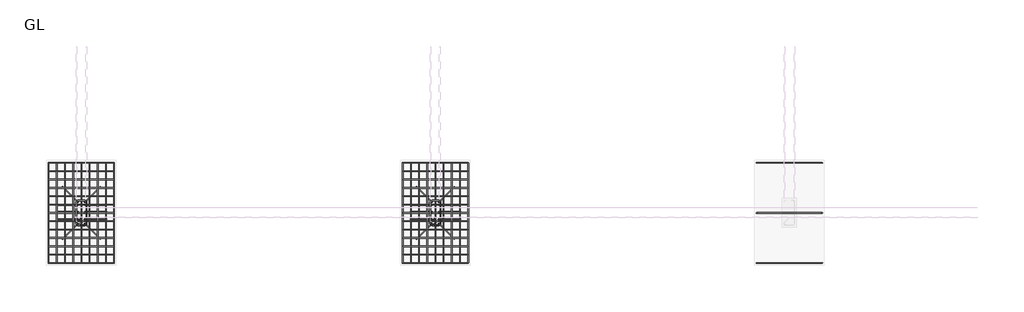
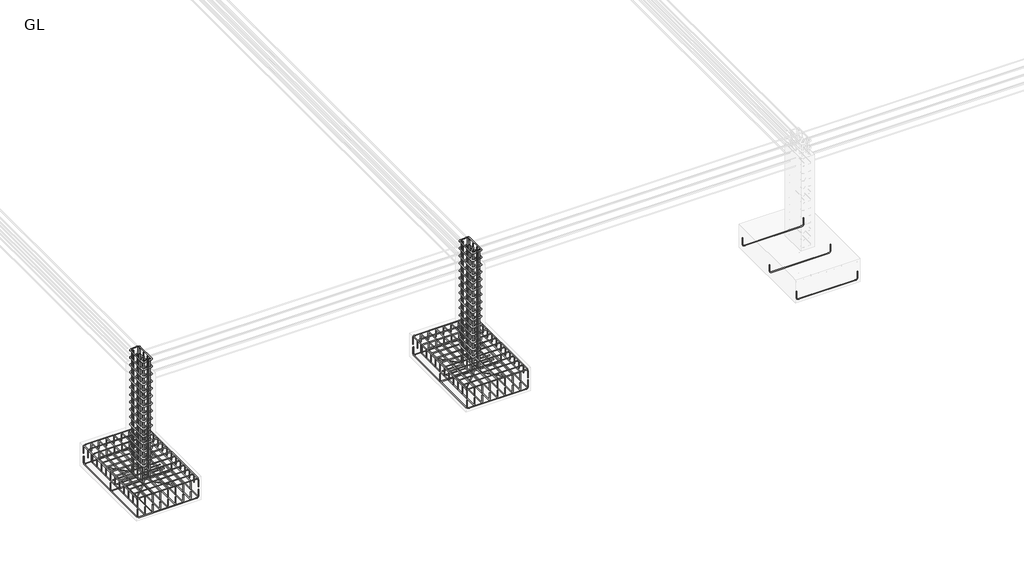
# One storey, part 2 of 16: 23 reinforcing bars.
"""IFC4 building model written with IfcOpenShell, lengths in millimetres."""

from ifc_helpers import new_model, si_unit, point, frame, origin, place, context, project, spatial, polyline, circle_curve, trimmed, segment, composite_curve, source, transform, mapped, element, save
from ifc_brep_helpers import swept_disk

model = new_model("IFC4")

# Units and contexts
model_context = context("Model", 3, world=origin())
ifc_project = project(units=[si_unit("LENGTHUNIT", "METRE", prefix="MILLI")], contexts=[model_context])

# Site, building, storey
site = spatial("IfcSite", under=ifc_project)
building = spatial("IfcBuilding", under=site)
storey = spatial("IfcBuildingStorey", under=building, Name="GL", Elevation=-1829.0)

# Reinforcing bars
placement = place(None, origin())
reinforcing_bar_shape = source(origin(), model_context, "Body", "SolidModel", [
    swept_disk(composite_curve([segment(polyline([(-22242.9544379, -19415.1167521, -2089.0), (-22242.9544379, -19415.1167521, -2213.0)]), True, "CONTINUOUS"), segment(trimmed(circle_curve(frame((-22272.9544379, -19415.1167521, -2213.0), z_axis=(0.0, 1.0, 0.0), x_axis=(30.0, 0.0, 0.0)), 30.0), [point((-22242.9544379, -19415.1167521, -2213.0))], [point((-22272.9544379, -19415.1167521, -2243.0))], True, "CARTESIAN"), True, "CONTINUOUS"), segment(polyline([(-22272.9544379, -19415.1167521, -2243.0), (-23340.9544379, -19415.1167521, -2243.0)]), True, "CONTINUOUS"), segment(trimmed(circle_curve(frame((-23340.9544379, -19415.1167521, -2213.0), z_axis=(0.0, 1.0, 0.0), x_axis=(0.0, 0.0, -30.0)), 30.0), [point((-23340.9544379, -19415.1167521, -2243.0))], [point((-23370.9544379, -19415.1167521, -2213.0))], True, "CARTESIAN"), True, "CONTINUOUS"), segment(polyline([(-23370.9544379, -19415.1167521, -2213.0), (-23370.9544379, -19415.1167521, -2089.0)]), True, "CONTINUOUS")], self_intersect=False), 6.0),
])
element("IfcReinforcingBar", 1, at=placement, inside=storey, context=model_context, shape_type="MappedRepresentation", body=[
    mapped(reinforcing_bar_shape, transform((0.0, 0.0, 0.0), x_axis=(1.0, 0.0, 0.0), y_axis=(0.0, 1.0, 0.0), z_axis=(0.0, 0.0, 1.0))),
    mapped(reinforcing_bar_shape, transform((0.0, -864.0, 0.0), x_axis=(1.0, 0.0, 0.0), y_axis=(0.0, 1.0, 0.0), z_axis=(0.0, 0.0, 1.0))),
    mapped(reinforcing_bar_shape, transform((0.0, -1728.0, 0.0), x_axis=(1.0, 0.0, 0.0), y_axis=(0.0, 1.0, 0.0), z_axis=(0.0, 0.0, 1.0))),
])
reinforcing_bar_2_shape = source(origin(), model_context, "Body", "SolidModel", [
    swept_disk(composite_curve([segment(polyline([(-23370.9544379, -19415.1167521, -2022.436678), (-23370.9544379, -19415.1167521, -1898.436678)]), True, "CONTINUOUS"), segment(trimmed(circle_curve(frame((-23340.9544379, -19415.1167521, -1898.436678), z_axis=(0.0, 1.0, 0.0), x_axis=(-30.0, 0.0, 0.0)), 30.0), [point((-23370.9544379, -19415.1167521, -1898.436678))], [point((-23340.9544379, -19415.1167521, -1868.436678))], True, "CARTESIAN"), True, "CONTINUOUS"), segment(polyline([(-23340.9544379, -19415.1167521, -1868.436678), (-22272.9544379, -19415.1167521, -1868.436678)]), True, "CONTINUOUS"), segment(trimmed(circle_curve(frame((-22272.9544379, -19415.1167521, -1898.436678), z_axis=(0.0, 1.0, 0.0), x_axis=(0.0, 0.0, 30.0)), 30.0), [point((-22272.9544379, -19415.1167521, -1868.436678))], [point((-22242.9544379, -19415.1167521, -1898.436678))], True, "CARTESIAN"), True, "CONTINUOUS"), segment(polyline([(-22242.9544379, -19415.1167521, -1898.436678), (-22242.9544379, -19415.1167521, -2022.436678)]), True, "CONTINUOUS")], self_intersect=False), 6.0),
])
element("IfcReinforcingBar", 2, at=placement, inside=storey, context=model_context, shape_type="MappedRepresentation", body=[
    mapped(reinforcing_bar_2_shape, transform((0.0, 0.0, 0.0), x_axis=(1.0, 0.0, 0.0), y_axis=(0.0, 1.0, 0.0), z_axis=(0.0, 0.0, 1.0))),
    mapped(reinforcing_bar_2_shape, transform((0.0, -144.0, 0.0), x_axis=(1.0, 0.0, 0.0), y_axis=(0.0, 1.0, 0.0), z_axis=(0.0, 0.0, 1.0))),
    mapped(reinforcing_bar_2_shape, transform((0.0, -288.0, 0.0), x_axis=(1.0, 0.0, 0.0), y_axis=(0.0, 1.0, 0.0), z_axis=(0.0, 0.0, 1.0))),
    mapped(reinforcing_bar_2_shape, transform((0.0, -432.0, 0.0), x_axis=(1.0, 0.0, 0.0), y_axis=(0.0, 1.0, 0.0), z_axis=(0.0, 0.0, 1.0))),
    mapped(reinforcing_bar_2_shape, transform((0.0, -576.0, 0.0), x_axis=(1.0, 0.0, 0.0), y_axis=(0.0, 1.0, 0.0), z_axis=(0.0, 0.0, 1.0))),
    mapped(reinforcing_bar_2_shape, transform((0.0, -720.0, 0.0), x_axis=(1.0, 0.0, 0.0), y_axis=(0.0, 1.0, 0.0), z_axis=(0.0, 0.0, 1.0))),
    mapped(reinforcing_bar_2_shape, transform((0.0, -864.0, 0.0), x_axis=(1.0, 0.0, 0.0), y_axis=(0.0, 1.0, 0.0), z_axis=(0.0, 0.0, 1.0))),
    mapped(reinforcing_bar_2_shape, transform((0.0, -1008.0, 0.0), x_axis=(1.0, 0.0, 0.0), y_axis=(0.0, 1.0, 0.0), z_axis=(0.0, 0.0, 1.0))),
    mapped(reinforcing_bar_2_shape, transform((0.0, -1152.0, 0.0), x_axis=(1.0, 0.0, 0.0), y_axis=(0.0, 1.0, 0.0), z_axis=(0.0, 0.0, 1.0))),
    mapped(reinforcing_bar_2_shape, transform((0.0, -1296.0, 0.0), x_axis=(1.0, 0.0, 0.0), y_axis=(0.0, 1.0, 0.0), z_axis=(0.0, 0.0, 1.0))),
    mapped(reinforcing_bar_2_shape, transform((0.0, -1440.0, 0.0), x_axis=(1.0, 0.0, 0.0), y_axis=(0.0, 1.0, 0.0), z_axis=(0.0, 0.0, 1.0))),
    mapped(reinforcing_bar_2_shape, transform((0.0, -1584.0, 0.0), x_axis=(1.0, 0.0, 0.0), y_axis=(0.0, 1.0, 0.0), z_axis=(0.0, 0.0, 1.0))),
    mapped(reinforcing_bar_2_shape, transform((0.0, -1728.0, 0.0), x_axis=(1.0, 0.0, 0.0), y_axis=(0.0, 1.0, 0.0), z_axis=(0.0, 0.0, 1.0))),
])
reinforcing_bar_3_shape = source(origin(), model_context, "Body", "SolidModel", [
    swept_disk(composite_curve([segment(polyline([(-23370.9544379, -21143.1167521, -2027.5081232), (-23370.9544379, -21143.1167521, -1903.5081232)]), True, "CONTINUOUS"), segment(trimmed(circle_curve(frame((-23370.9544379, -21113.1167521, -1903.5081232), z_axis=(-1.0, 0.0, 0.0), x_axis=(0.0, -30.0, 0.0)), 30.0), [point((-23370.9544379, -21143.1167521, -1903.5081232))], [point((-23370.9544379, -21113.1167521, -1873.5081232))], True, "CARTESIAN"), True, "CONTINUOUS"), segment(polyline([(-23370.9544379, -21113.1167521, -1873.5081232), (-23370.9544379, -19445.1167521, -1873.5081232)]), True, "CONTINUOUS"), segment(trimmed(circle_curve(frame((-23370.9544379, -19445.1167521, -1903.5081232), z_axis=(-1.0, 0.0, 0.0), x_axis=(0.0, 0.0, 30.0)), 30.0), [point((-23370.9544379, -19445.1167521, -1873.5081232))], [point((-23370.9544379, -19415.1167521, -1903.5081232))], True, "CARTESIAN"), True, "CONTINUOUS"), segment(polyline([(-23370.9544379, -19415.1167521, -1903.5081232), (-23370.9544379, -19415.1167521, -2027.5081232)]), True, "CONTINUOUS")], self_intersect=False), 6.0),
])
element("IfcReinforcingBar", 3, at=placement, inside=storey, context=model_context, shape_type="MappedRepresentation", body=[
    mapped(reinforcing_bar_3_shape, transform((0.0, 0.0, 0.0), x_axis=(1.0, 0.0, 0.0), y_axis=(0.0, 1.0, 0.0), z_axis=(0.0, 0.0, 1.0))),
    mapped(reinforcing_bar_3_shape, transform((141.0, 0.0, 0.0), x_axis=(1.0, 0.0, 0.0), y_axis=(0.0, 1.0, 0.0), z_axis=(0.0, 0.0, 1.0))),
    mapped(reinforcing_bar_3_shape, transform((282.0, 0.0, 0.0), x_axis=(1.0, 0.0, 0.0), y_axis=(0.0, 1.0, 0.0), z_axis=(0.0, 0.0, 1.0))),
    mapped(reinforcing_bar_3_shape, transform((423.0, 0.0, 0.0), x_axis=(1.0, 0.0, 0.0), y_axis=(0.0, 1.0, 0.0), z_axis=(0.0, 0.0, 1.0))),
    mapped(reinforcing_bar_3_shape, transform((564.0, 0.0, 0.0), x_axis=(1.0, 0.0, 0.0), y_axis=(0.0, 1.0, 0.0), z_axis=(0.0, 0.0, 1.0))),
    mapped(reinforcing_bar_3_shape, transform((705.0, 0.0, 0.0), x_axis=(1.0, 0.0, 0.0), y_axis=(0.0, 1.0, 0.0), z_axis=(0.0, 0.0, 1.0))),
    mapped(reinforcing_bar_3_shape, transform((846.0, 0.0, 0.0), x_axis=(1.0, 0.0, 0.0), y_axis=(0.0, 1.0, 0.0), z_axis=(0.0, 0.0, 1.0))),
    mapped(reinforcing_bar_3_shape, transform((987.0, 0.0, 0.0), x_axis=(1.0, 0.0, 0.0), y_axis=(0.0, 1.0, 0.0), z_axis=(0.0, 0.0, 1.0))),
    mapped(reinforcing_bar_3_shape, transform((1128.0, 0.0, 0.0), x_axis=(1.0, 0.0, 0.0), y_axis=(0.0, 1.0, 0.0), z_axis=(0.0, 0.0, 1.0))),
])
reinforcing_bar_4_shape = source(origin(), model_context, "Body", "SolidModel", [
    swept_disk(composite_curve([segment(polyline([(-22242.9544379, -21143.1167521, -2080.6239909), (-22242.9544379, -21143.1167521, -2204.6239909)]), True, "CONTINUOUS"), segment(trimmed(circle_curve(frame((-22242.9544379, -21113.1167521, -2204.6239909), z_axis=(1.0, 0.0, 0.0), x_axis=(0.0, -30.0, 0.0)), 30.0), [point((-22242.9544379, -21143.1167521, -2204.6239909))], [point((-22242.9544379, -21113.1167521, -2234.6239909))], True, "CARTESIAN"), True, "CONTINUOUS"), segment(polyline([(-22242.9544379, -21113.1167521, -2234.6239909), (-22242.9544379, -19458.1421892, -2234.6239909)]), True, "CONTINUOUS"), segment(trimmed(circle_curve(frame((-22242.9544379, -19458.1421892, -2204.6239909), z_axis=(1.0, 0.0, 0.0), x_axis=(0.0, 0.0, -30.0)), 30.0), [point((-22242.9544379, -19458.1421892, -2234.6239909))], [point((-22242.9544379, -19428.1421892, -2204.6239909))], True, "CARTESIAN"), True, "CONTINUOUS"), segment(polyline([(-22242.9544379, -19428.1421892, -2204.6239909), (-22242.9544379, -19428.1421892, -2080.6239909)]), True, "CONTINUOUS")], self_intersect=False), 6.0),
])
element("IfcReinforcingBar", 4, at=placement, inside=storey, context=model_context, shape_type="MappedRepresentation", body=[
    mapped(reinforcing_bar_4_shape, transform((0.0, 0.0, 0.0), x_axis=(1.0, 0.0, 0.0), y_axis=(0.0, 1.0, 0.0), z_axis=(0.0, 0.0, 1.0))),
    mapped(reinforcing_bar_4_shape, transform((-141.0, 0.0, 0.0), x_axis=(1.0, 0.0, 0.0), y_axis=(0.0, 1.0, 0.0), z_axis=(0.0, 0.0, 1.0))),
    mapped(reinforcing_bar_4_shape, transform((-282.0, 0.0, 0.0), x_axis=(1.0, 0.0, 0.0), y_axis=(0.0, 1.0, 0.0), z_axis=(0.0, 0.0, 1.0))),
    mapped(reinforcing_bar_4_shape, transform((-423.0, 0.0, 0.0), x_axis=(1.0, 0.0, 0.0), y_axis=(0.0, 1.0, 0.0), z_axis=(0.0, 0.0, 1.0))),
    mapped(reinforcing_bar_4_shape, transform((-564.0, 0.0, 0.0), x_axis=(1.0, 0.0, 0.0), y_axis=(0.0, 1.0, 0.0), z_axis=(0.0, 0.0, 1.0))),
    mapped(reinforcing_bar_4_shape, transform((-705.0, 0.0, 0.0), x_axis=(1.0, 0.0, 0.0), y_axis=(0.0, 1.0, 0.0), z_axis=(0.0, 0.0, 1.0))),
    mapped(reinforcing_bar_4_shape, transform((-846.0, 0.0, 0.0), x_axis=(1.0, 0.0, 0.0), y_axis=(0.0, 1.0, 0.0), z_axis=(0.0, 0.0, 1.0))),
    mapped(reinforcing_bar_4_shape, transform((-987.0, 0.0, 0.0), x_axis=(1.0, 0.0, 0.0), y_axis=(0.0, 1.0, 0.0), z_axis=(0.0, 0.0, 1.0))),
    mapped(reinforcing_bar_4_shape, transform((-1128.0, 0.0, 0.0), x_axis=(1.0, 0.0, 0.0), y_axis=(0.0, 1.0, 0.0), z_axis=(0.0, 0.0, 1.0))),
])
reinforcing_bar_5_shape = source(origin(), model_context, "Body", "SolidModel", [
    swept_disk(composite_curve([segment(polyline([(-16146.9544379, -19415.1167521, -2089.0), (-16146.9544379, -19415.1167521, -2213.0)]), True, "CONTINUOUS"), segment(trimmed(circle_curve(frame((-16176.9544379, -19415.1167521, -2213.0), z_axis=(0.0, 1.0, 0.0), x_axis=(30.0, 0.0, 0.0)), 30.0), [point((-16146.9544379, -19415.1167521, -2213.0))], [point((-16176.9544379, -19415.1167521, -2243.0))], True, "CARTESIAN"), True, "CONTINUOUS"), segment(polyline([(-16176.9544379, -19415.1167521, -2243.0), (-17244.9544379, -19415.1167521, -2243.0)]), True, "CONTINUOUS"), segment(trimmed(circle_curve(frame((-17244.9544379, -19415.1167521, -2213.0), z_axis=(0.0, 1.0, 0.0), x_axis=(0.0, 0.0, -30.0)), 30.0), [point((-17244.9544379, -19415.1167521, -2243.0))], [point((-17274.9544379, -19415.1167521, -2213.0))], True, "CARTESIAN"), True, "CONTINUOUS"), segment(polyline([(-17274.9544379, -19415.1167521, -2213.0), (-17274.9544379, -19415.1167521, -2089.0)]), True, "CONTINUOUS")], self_intersect=False), 6.0),
])
element("IfcReinforcingBar", 5, at=placement, inside=storey, context=model_context, shape_type="MappedRepresentation", body=[
    mapped(reinforcing_bar_5_shape, transform((0.0, 0.0, 0.0), x_axis=(1.0, 0.0, 0.0), y_axis=(0.0, 1.0, 0.0), z_axis=(0.0, 0.0, 1.0))),
    mapped(reinforcing_bar_5_shape, transform((0.0, -864.0, 0.0), x_axis=(1.0, 0.0, 0.0), y_axis=(0.0, 1.0, 0.0), z_axis=(0.0, 0.0, 1.0))),
    mapped(reinforcing_bar_5_shape, transform((0.0, -1728.0, 0.0), x_axis=(1.0, 0.0, 0.0), y_axis=(0.0, 1.0, 0.0), z_axis=(0.0, 0.0, 1.0))),
])
reinforcing_bar_6_shape = source(origin(), model_context, "Body", "SolidModel", [
    swept_disk(composite_curve([segment(polyline([(-17274.9544379, -19415.1167521, -2022.436678), (-17274.9544379, -19415.1167521, -1898.436678)]), True, "CONTINUOUS"), segment(trimmed(circle_curve(frame((-17244.9544379, -19415.1167521, -1898.436678), z_axis=(0.0, 1.0, 0.0), x_axis=(-30.0, 0.0, 0.0)), 30.0), [point((-17274.9544379, -19415.1167521, -1898.436678))], [point((-17244.9544379, -19415.1167521, -1868.436678))], True, "CARTESIAN"), True, "CONTINUOUS"), segment(polyline([(-17244.9544379, -19415.1167521, -1868.436678), (-16176.9544379, -19415.1167521, -1868.436678)]), True, "CONTINUOUS"), segment(trimmed(circle_curve(frame((-16176.9544379, -19415.1167521, -1898.436678), z_axis=(0.0, 1.0, 0.0), x_axis=(0.0, 0.0, 30.0)), 30.0), [point((-16176.9544379, -19415.1167521, -1868.436678))], [point((-16146.9544379, -19415.1167521, -1898.436678))], True, "CARTESIAN"), True, "CONTINUOUS"), segment(polyline([(-16146.9544379, -19415.1167521, -1898.436678), (-16146.9544379, -19415.1167521, -2022.436678)]), True, "CONTINUOUS")], self_intersect=False), 6.0),
])
element("IfcReinforcingBar", 6, at=placement, inside=storey, context=model_context, shape_type="MappedRepresentation", body=[
    mapped(reinforcing_bar_6_shape, transform((0.0, 0.0, 0.0), x_axis=(1.0, 0.0, 0.0), y_axis=(0.0, 1.0, 0.0), z_axis=(0.0, 0.0, 1.0))),
    mapped(reinforcing_bar_6_shape, transform((0.0, -144.0, 0.0), x_axis=(1.0, 0.0, 0.0), y_axis=(0.0, 1.0, 0.0), z_axis=(0.0, 0.0, 1.0))),
    mapped(reinforcing_bar_6_shape, transform((0.0, -288.0, 0.0), x_axis=(1.0, 0.0, 0.0), y_axis=(0.0, 1.0, 0.0), z_axis=(0.0, 0.0, 1.0))),
    mapped(reinforcing_bar_6_shape, transform((0.0, -432.0, 0.0), x_axis=(1.0, 0.0, 0.0), y_axis=(0.0, 1.0, 0.0), z_axis=(0.0, 0.0, 1.0))),
    mapped(reinforcing_bar_6_shape, transform((0.0, -576.0, 0.0), x_axis=(1.0, 0.0, 0.0), y_axis=(0.0, 1.0, 0.0), z_axis=(0.0, 0.0, 1.0))),
    mapped(reinforcing_bar_6_shape, transform((0.0, -720.0, 0.0), x_axis=(1.0, 0.0, 0.0), y_axis=(0.0, 1.0, 0.0), z_axis=(0.0, 0.0, 1.0))),
    mapped(reinforcing_bar_6_shape, transform((0.0, -864.0, 0.0), x_axis=(1.0, 0.0, 0.0), y_axis=(0.0, 1.0, 0.0), z_axis=(0.0, 0.0, 1.0))),
    mapped(reinforcing_bar_6_shape, transform((0.0, -1008.0, 0.0), x_axis=(1.0, 0.0, 0.0), y_axis=(0.0, 1.0, 0.0), z_axis=(0.0, 0.0, 1.0))),
    mapped(reinforcing_bar_6_shape, transform((0.0, -1152.0, 0.0), x_axis=(1.0, 0.0, 0.0), y_axis=(0.0, 1.0, 0.0), z_axis=(0.0, 0.0, 1.0))),
    mapped(reinforcing_bar_6_shape, transform((0.0, -1296.0, 0.0), x_axis=(1.0, 0.0, 0.0), y_axis=(0.0, 1.0, 0.0), z_axis=(0.0, 0.0, 1.0))),
    mapped(reinforcing_bar_6_shape, transform((0.0, -1440.0, 0.0), x_axis=(1.0, 0.0, 0.0), y_axis=(0.0, 1.0, 0.0), z_axis=(0.0, 0.0, 1.0))),
    mapped(reinforcing_bar_6_shape, transform((0.0, -1584.0, 0.0), x_axis=(1.0, 0.0, 0.0), y_axis=(0.0, 1.0, 0.0), z_axis=(0.0, 0.0, 1.0))),
    mapped(reinforcing_bar_6_shape, transform((0.0, -1728.0, 0.0), x_axis=(1.0, 0.0, 0.0), y_axis=(0.0, 1.0, 0.0), z_axis=(0.0, 0.0, 1.0))),
])
reinforcing_bar_7_shape = source(origin(), model_context, "Body", "SolidModel", [
    swept_disk(composite_curve([segment(polyline([(-17274.9544379, -21143.1167521, -2027.5081232), (-17274.9544379, -21143.1167521, -1903.5081232)]), True, "CONTINUOUS"), segment(trimmed(circle_curve(frame((-17274.9544379, -21113.1167521, -1903.5081232), z_axis=(-1.0, 0.0, 0.0), x_axis=(0.0, -30.0, 0.0)), 30.0), [point((-17274.9544379, -21143.1167521, -1903.5081232))], [point((-17274.9544379, -21113.1167521, -1873.5081232))], True, "CARTESIAN"), True, "CONTINUOUS"), segment(polyline([(-17274.9544379, -21113.1167521, -1873.5081232), (-17274.9544379, -19445.1167521, -1873.5081232)]), True, "CONTINUOUS"), segment(trimmed(circle_curve(frame((-17274.9544379, -19445.1167521, -1903.5081232), z_axis=(-1.0, 0.0, 0.0), x_axis=(0.0, 0.0, 30.0)), 30.0), [point((-17274.9544379, -19445.1167521, -1873.5081232))], [point((-17274.9544379, -19415.1167521, -1903.5081232))], True, "CARTESIAN"), True, "CONTINUOUS"), segment(polyline([(-17274.9544379, -19415.1167521, -1903.5081232), (-17274.9544379, -19415.1167521, -2027.5081232)]), True, "CONTINUOUS")], self_intersect=False), 6.0),
])
element("IfcReinforcingBar", 7, at=placement, inside=storey, context=model_context, shape_type="MappedRepresentation", body=[
    mapped(reinforcing_bar_7_shape, transform((0.0, 0.0, 0.0), x_axis=(1.0, 0.0, 0.0), y_axis=(0.0, 1.0, 0.0), z_axis=(0.0, 0.0, 1.0))),
    mapped(reinforcing_bar_7_shape, transform((141.0, 0.0, 0.0), x_axis=(1.0, 0.0, 0.0), y_axis=(0.0, 1.0, 0.0), z_axis=(0.0, 0.0, 1.0))),
    mapped(reinforcing_bar_7_shape, transform((282.0, 0.0, 0.0), x_axis=(1.0, 0.0, 0.0), y_axis=(0.0, 1.0, 0.0), z_axis=(0.0, 0.0, 1.0))),
    mapped(reinforcing_bar_7_shape, transform((423.0, 0.0, 0.0), x_axis=(1.0, 0.0, 0.0), y_axis=(0.0, 1.0, 0.0), z_axis=(0.0, 0.0, 1.0))),
    mapped(reinforcing_bar_7_shape, transform((564.0, 0.0, 0.0), x_axis=(1.0, 0.0, 0.0), y_axis=(0.0, 1.0, 0.0), z_axis=(0.0, 0.0, 1.0))),
    mapped(reinforcing_bar_7_shape, transform((705.0, 0.0, 0.0), x_axis=(1.0, 0.0, 0.0), y_axis=(0.0, 1.0, 0.0), z_axis=(0.0, 0.0, 1.0))),
    mapped(reinforcing_bar_7_shape, transform((846.0, 0.0, 0.0), x_axis=(1.0, 0.0, 0.0), y_axis=(0.0, 1.0, 0.0), z_axis=(0.0, 0.0, 1.0))),
    mapped(reinforcing_bar_7_shape, transform((987.0, 0.0, 0.0), x_axis=(1.0, 0.0, 0.0), y_axis=(0.0, 1.0, 0.0), z_axis=(0.0, 0.0, 1.0))),
    mapped(reinforcing_bar_7_shape, transform((1128.0, 0.0, 0.0), x_axis=(1.0, 0.0, 0.0), y_axis=(0.0, 1.0, 0.0), z_axis=(0.0, 0.0, 1.0))),
])
reinforcing_bar_8_shape = source(origin(), model_context, "Body", "SolidModel", [
    swept_disk(composite_curve([segment(polyline([(-16146.9544379, -21143.1167521, -2080.6239909), (-16146.9544379, -21143.1167521, -2204.6239909)]), True, "CONTINUOUS"), segment(trimmed(circle_curve(frame((-16146.9544379, -21113.1167521, -2204.6239909), z_axis=(1.0, 0.0, 0.0), x_axis=(0.0, -30.0, 0.0)), 30.0), [point((-16146.9544379, -21143.1167521, -2204.6239909))], [point((-16146.9544379, -21113.1167521, -2234.6239909))], True, "CARTESIAN"), True, "CONTINUOUS"), segment(polyline([(-16146.9544379, -21113.1167521, -2234.6239909), (-16146.9544379, -19458.1421892, -2234.6239909)]), True, "CONTINUOUS"), segment(trimmed(circle_curve(frame((-16146.9544379, -19458.1421892, -2204.6239909), z_axis=(1.0, 0.0, 0.0), x_axis=(0.0, 0.0, -30.0)), 30.0), [point((-16146.9544379, -19458.1421892, -2234.6239909))], [point((-16146.9544379, -19428.1421892, -2204.6239909))], True, "CARTESIAN"), True, "CONTINUOUS"), segment(polyline([(-16146.9544379, -19428.1421892, -2204.6239909), (-16146.9544379, -19428.1421892, -2080.6239909)]), True, "CONTINUOUS")], self_intersect=False), 6.0),
])
element("IfcReinforcingBar", 8, at=placement, inside=storey, context=model_context, shape_type="MappedRepresentation", body=[
    mapped(reinforcing_bar_8_shape, transform((0.0, 0.0, 0.0), x_axis=(1.0, 0.0, 0.0), y_axis=(0.0, 1.0, 0.0), z_axis=(0.0, 0.0, 1.0))),
    mapped(reinforcing_bar_8_shape, transform((-141.0, 0.0, 0.0), x_axis=(1.0, 0.0, 0.0), y_axis=(0.0, 1.0, 0.0), z_axis=(0.0, 0.0, 1.0))),
    mapped(reinforcing_bar_8_shape, transform((-282.0, 0.0, 0.0), x_axis=(1.0, 0.0, 0.0), y_axis=(0.0, 1.0, 0.0), z_axis=(0.0, 0.0, 1.0))),
    mapped(reinforcing_bar_8_shape, transform((-423.0, 0.0, 0.0), x_axis=(1.0, 0.0, 0.0), y_axis=(0.0, 1.0, 0.0), z_axis=(0.0, 0.0, 1.0))),
    mapped(reinforcing_bar_8_shape, transform((-564.0, 0.0, 0.0), x_axis=(1.0, 0.0, 0.0), y_axis=(0.0, 1.0, 0.0), z_axis=(0.0, 0.0, 1.0))),
    mapped(reinforcing_bar_8_shape, transform((-705.0, 0.0, 0.0), x_axis=(1.0, 0.0, 0.0), y_axis=(0.0, 1.0, 0.0), z_axis=(0.0, 0.0, 1.0))),
    mapped(reinforcing_bar_8_shape, transform((-846.0, 0.0, 0.0), x_axis=(1.0, 0.0, 0.0), y_axis=(0.0, 1.0, 0.0), z_axis=(0.0, 0.0, 1.0))),
    mapped(reinforcing_bar_8_shape, transform((-987.0, 0.0, 0.0), x_axis=(1.0, 0.0, 0.0), y_axis=(0.0, 1.0, 0.0), z_axis=(0.0, 0.0, 1.0))),
    mapped(reinforcing_bar_8_shape, transform((-1128.0, 0.0, 0.0), x_axis=(1.0, 0.0, 0.0), y_axis=(0.0, 1.0, 0.0), z_axis=(0.0, 0.0, 1.0))),
])
reinforcing_bar_9_shape = source(origin(), model_context, "Body", "SolidModel", [
    swept_disk(composite_curve([segment(polyline([(-10050.9544379, -19415.1167521, -2089.0), (-10050.9544379, -19415.1167521, -2213.0)]), True, "CONTINUOUS"), segment(trimmed(circle_curve(frame((-10080.9544379, -19415.1167521, -2213.0), z_axis=(0.0, 1.0, 0.0), x_axis=(30.0, 0.0, 0.0)), 30.0), [point((-10050.9544379, -19415.1167521, -2213.0))], [point((-10080.9544379, -19415.1167521, -2243.0))], True, "CARTESIAN"), True, "CONTINUOUS"), segment(polyline([(-10080.9544379, -19415.1167521, -2243.0), (-11148.9544379, -19415.1167521, -2243.0)]), True, "CONTINUOUS"), segment(trimmed(circle_curve(frame((-11148.9544379, -19415.1167521, -2213.0), z_axis=(0.0, 1.0, 0.0), x_axis=(0.0, 0.0, -30.0)), 30.0), [point((-11148.9544379, -19415.1167521, -2243.0))], [point((-11178.9544379, -19415.1167521, -2213.0))], True, "CARTESIAN"), True, "CONTINUOUS"), segment(polyline([(-11178.9544379, -19415.1167521, -2213.0), (-11178.9544379, -19415.1167521, -2089.0)]), True, "CONTINUOUS")], self_intersect=False), 6.0),
])
element("IfcReinforcingBar", 9, at=placement, inside=storey, context=model_context, shape_type="MappedRepresentation", body=[
    mapped(reinforcing_bar_9_shape, transform((0.0, 0.0, 0.0), x_axis=(1.0, 0.0, 0.0), y_axis=(0.0, 1.0, 0.0), z_axis=(0.0, 0.0, 1.0))),
    mapped(reinforcing_bar_9_shape, transform((0.0, -864.0, 0.0), x_axis=(1.0, 0.0, 0.0), y_axis=(0.0, 1.0, 0.0), z_axis=(0.0, 0.0, 1.0))),
    mapped(reinforcing_bar_9_shape, transform((0.0, -1728.0, 0.0), x_axis=(1.0, 0.0, 0.0), y_axis=(0.0, 1.0, 0.0), z_axis=(0.0, 0.0, 1.0))),
])
reinforcing_bar_10_shape = source(origin(), model_context, "Body", "SolidModel", [
    swept_disk(composite_curve([segment(polyline([(-16703.4864005, -20354.2223078, -1793.0), (-16791.1676414, -20441.9035486, -1793.0)]), True, "CONTINUOUS"), segment(trimmed(circle_curve(frame((-16769.9544379, -20463.1167521, -1793.0), z_axis=(0.0, 0.0, 1.0), x_axis=(-21.21320349999951, 21.21320349999951, 0.0)), 30.0), [point((-16791.1676414, -20441.9035486, -1793.0))], [point((-16769.9544379, -20493.1167521, -1793.0))], True, "CARTESIAN"), True, "CONTINUOUS"), segment(polyline([(-16769.9544379, -20493.1167521, -1793.0), (-16651.9544379, -20493.1167521, -1793.0)]), True, "CONTINUOUS"), segment(trimmed(circle_curve(frame((-16651.9544379, -20463.1167521, -1793.0), z_axis=(0.0, 0.0, 1.0), x_axis=(0.0, -30.0, 0.0)), 30.0), [point((-16651.9544379, -20493.1167521, -1793.0))], [point((-16621.9544379, -20463.1167521, -1793.0))], True, "CARTESIAN"), True, "CONTINUOUS"), segment(polyline([(-16621.9544379, -20463.1167521, -1793.0), (-16621.9544379, -20095.1167521, -1793.0)]), True, "CONTINUOUS"), segment(trimmed(circle_curve(frame((-16651.8864962, -20095.1167521, -1795.0178916), z_axis=(-0.06726305234213417, 0.0, 0.9977352764083365), x_axis=(29.93205830000079, 0.0, 2.0178915999999845)), 30.0), [point((-16621.9544379, -20095.1167521, -1793.0))], [point((-16651.8864962, -20065.1167521, -1795.0178916))], True, "CARTESIAN"), True, "CONTINUOUS"), segment(polyline([(-16651.8864962, -20065.1167521, -1795.0178916), (-16770.0223796, -20065.1167521, -1802.9821084)]), True, "CONTINUOUS"), segment(trimmed(circle_curve(frame((-16770.0223796, -20095.1167521, -1802.9821084), z_axis=(-0.06726305234213417, 0.0, 0.9977352764083365), x_axis=(0.0, 30.0, 0.0)), 30.0), [point((-16770.0223796, -20065.1167521, -1802.9821084))], [point((-16799.9544379, -20095.1167521, -1805.0))], True, "CARTESIAN"), True, "CONTINUOUS"), segment(polyline([(-16799.9544379, -20095.1167521, -1805.0), (-16799.9544379, -20463.1167521, -1805.0)]), True, "CONTINUOUS"), segment(trimmed(circle_curve(frame((-16769.9544379, -20463.1167521, -1805.0), z_axis=(0.0, 0.0, 1.0), x_axis=(-30.0, 0.0, 0.0)), 30.0), [point((-16799.9544379, -20463.1167521, -1805.0))], [point((-16748.7412345, -20484.3299555, -1805.0))], True, "CARTESIAN"), True, "CONTINUOUS"), segment(polyline([(-16748.7412345, -20484.3299555, -1805.0), (-16661.0599936, -20396.6487146, -1805.0)]), True, "CONTINUOUS")], self_intersect=False), 6.0),
])
element("IfcReinforcingBar", 10, at=placement, inside=storey, context=model_context, shape_type="MappedRepresentation", body=[
    mapped(reinforcing_bar_10_shape, transform((0.0, 0.0, 0.0), x_axis=(1.0, 0.0, 0.0), y_axis=(0.0, 1.0, 0.0), z_axis=(0.0, 0.0, 1.0))),
    mapped(reinforcing_bar_10_shape, transform((0.0, 0.0, 144.8571429), x_axis=(1.0, 0.0, 0.0), y_axis=(0.0, 1.0, 0.0), z_axis=(0.0, 0.0, 1.0))),
    mapped(reinforcing_bar_10_shape, transform((0.0, 0.0, 289.7142857), x_axis=(1.0, 0.0, 0.0), y_axis=(0.0, 1.0, 0.0), z_axis=(0.0, 0.0, 1.0))),
    mapped(reinforcing_bar_10_shape, transform((0.0, 0.0, 434.5714286), x_axis=(1.0, 0.0, 0.0), y_axis=(0.0, 1.0, 0.0), z_axis=(0.0, 0.0, 1.0))),
    mapped(reinforcing_bar_10_shape, transform((0.0, 0.0, 579.4285714), x_axis=(1.0, 0.0, 0.0), y_axis=(0.0, 1.0, 0.0), z_axis=(0.0, 0.0, 1.0))),
    mapped(reinforcing_bar_10_shape, transform((0.0, 0.0, 724.2857143), x_axis=(1.0, 0.0, 0.0), y_axis=(0.0, 1.0, 0.0), z_axis=(0.0, 0.0, 1.0))),
    mapped(reinforcing_bar_10_shape, transform((0.0, 0.0, 869.1428571), x_axis=(1.0, 0.0, 0.0), y_axis=(0.0, 1.0, 0.0), z_axis=(0.0, 0.0, 1.0))),
    mapped(reinforcing_bar_10_shape, transform((0.0, 0.0, 1014.0), x_axis=(1.0, 0.0, 0.0), y_axis=(0.0, 1.0, 0.0), z_axis=(0.0, 0.0, 1.0))),
    mapped(reinforcing_bar_10_shape, transform((0.0, 0.0, 1158.8571429), x_axis=(1.0, 0.0, 0.0), y_axis=(0.0, 1.0, 0.0), z_axis=(0.0, 0.0, 1.0))),
    mapped(reinforcing_bar_10_shape, transform((0.0, 0.0, 1303.7142857), x_axis=(1.0, 0.0, 0.0), y_axis=(0.0, 1.0, 0.0), z_axis=(0.0, 0.0, 1.0))),
    mapped(reinforcing_bar_10_shape, transform((0.0, 0.0, 1448.5714286), x_axis=(1.0, 0.0, 0.0), y_axis=(0.0, 1.0, 0.0), z_axis=(0.0, 0.0, 1.0))),
    mapped(reinforcing_bar_10_shape, transform((0.0, 0.0, 1593.4285714), x_axis=(1.0, 0.0, 0.0), y_axis=(0.0, 1.0, 0.0), z_axis=(0.0, 0.0, 1.0))),
    mapped(reinforcing_bar_10_shape, transform((0.0, 0.0, 1738.2857143), x_axis=(1.0, 0.0, 0.0), y_axis=(0.0, 1.0, 0.0), z_axis=(0.0, 0.0, 1.0))),
    mapped(reinforcing_bar_10_shape, transform((0.0, 0.0, 1883.1428571), x_axis=(1.0, 0.0, 0.0), y_axis=(0.0, 1.0, 0.0), z_axis=(0.0, 0.0, 1.0))),
    mapped(reinforcing_bar_10_shape, transform((0.0, 0.0, 2028.0), x_axis=(1.0, 0.0, 0.0), y_axis=(0.0, 1.0, 0.0), z_axis=(0.0, 0.0, 1.0))),
])
element("IfcReinforcingBar", 11, at=placement, inside=storey, context=model_context, shape_type="SolidModel", body=[
    swept_disk(composite_curve([segment(polyline([(-16768.0642232, -20464.0642439, 241.0), (-16768.0642232, -20464.0642439, -2129.0)]), True, "CONTINUOUS"), segment(trimmed(circle_curve(frame((-16789.2774266, -20485.2774473, -2129.0), z_axis=(-0.7071067811865187, 0.7071067811865764, 0.0), x_axis=(21.213203400002385, 21.213203399998747, 0.0)), 30.0), [point((-16768.0642232, -20464.0642439, -2129.0))], [point((-16789.2774266, -20485.2774473, -2159.0))], True, "CARTESIAN"), True, "CONTINUOUS"), segment(polyline([(-16789.2774266, -20485.2774473, -2159.0), (-17036.7648, -20732.7648207, -2159.0)]), True, "CONTINUOUS")], self_intersect=False), 6.0),
])
element("IfcReinforcingBar", 12, at=placement, inside=storey, context=model_context, shape_type="SolidModel", body=[
    swept_disk(composite_curve([segment(polyline([(-16768.0642232, -20094.1692603, 241.0), (-16768.0642232, -20094.1692603, -2129.0)]), True, "CONTINUOUS"), segment(trimmed(circle_curve(frame((-16789.2774266, -20072.9560568, -2129.0), z_axis=(0.7071067811865218, 0.7071067811865733, 0.0), x_axis=(21.213203400002385, -21.21320349999951, 0.0)), 30.0), [point((-16768.0642232, -20094.1692603, -2129.0))], [point((-16789.2774266, -20072.9560568, -2159.0))], True, "CARTESIAN"), True, "CONTINUOUS"), segment(polyline([(-16789.2774266, -20072.9560568, -2159.0), (-17036.7648, -19825.4686834, -2159.0)]), True, "CONTINUOUS")], self_intersect=False), 6.0),
])
element("IfcReinforcingBar", 13, at=placement, inside=storey, context=model_context, shape_type="SolidModel", body=[
    swept_disk(composite_curve([segment(polyline([(-16653.8446527, -20464.0642439, 241.0), (-16653.8446527, -20464.0642439, -2129.0)]), True, "CONTINUOUS"), segment(trimmed(circle_curve(frame((-16632.6314492, -20485.2774473, -2129.0), z_axis=(-0.7071067811865248, -0.7071067811865703, 0.0), x_axis=(-21.213203500003146, 21.213203399998747, 0.0)), 30.0), [point((-16653.8446527, -20464.0642439, -2129.0))], [point((-16632.6314492, -20485.2774473, -2159.0))], True, "CARTESIAN"), True, "CONTINUOUS"), segment(polyline([(-16632.6314492, -20485.2774473, -2159.0), (-16385.1440758, -20732.7648207, -2159.0)]), True, "CONTINUOUS")], self_intersect=False), 6.0),
])
element("IfcReinforcingBar", 14, at=placement, inside=storey, context=model_context, shape_type="SolidModel", body=[
    swept_disk(composite_curve([segment(polyline([(-16653.8446527, -20094.1692603, 241.0), (-16653.8446527, -20094.1692603, -2129.0)]), True, "CONTINUOUS"), segment(trimmed(circle_curve(frame((-16632.6314492, -20072.9560568, -2129.0), z_axis=(0.7071067811865157, -0.7071067811865794, 0.0), x_axis=(-21.213203500003146, -21.21320349999951, 0.0)), 30.0), [point((-16653.8446527, -20094.1692603, -2129.0))], [point((-16632.6314492, -20072.9560568, -2159.0))], True, "CARTESIAN"), True, "CONTINUOUS"), segment(polyline([(-16632.6314492, -20072.9560568, -2159.0), (-16385.1440758, -19825.4686834, -2159.0)]), True, "CONTINUOUS")], self_intersect=False), 6.0),
])
reinforcing_bar_11_shape = source(origin(), model_context, "Body", "SolidModel", [
    swept_disk(composite_curve([segment(polyline([(-16768.0642232, -20386.9117405, 241.0), (-16768.0642232, -20386.9117405, -2129.0)]), True, "CONTINUOUS"), segment(trimmed(circle_curve(frame((-16798.0642232, -20386.9117405, -2129.0), z_axis=(0.0, 1.0, 0.0), x_axis=(30.0, 0.0, 0.0)), 30.0), [point((-16768.0642232, -20386.9117405, -2129.0))], [point((-16798.0642232, -20386.9117405, -2159.0))], True, "CARTESIAN"), True, "CONTINUOUS"), segment(polyline([(-16798.0642232, -20386.9117405, -2159.0), (-17148.0642232, -20386.9117405, -2159.0)]), True, "CONTINUOUS")], self_intersect=False), 6.0),
])
element("IfcReinforcingBar", 15, at=placement, inside=storey, context=model_context, shape_type="MappedRepresentation", body=[
    mapped(reinforcing_bar_11_shape, transform((0.0, 0.0, 0.0), x_axis=(1.0, 0.0, 0.0), y_axis=(0.0, 1.0, 0.0), z_axis=(0.0, 0.0, 1.0))),
    mapped(reinforcing_bar_11_shape, transform((0.0, 123.5823926, 0.0), x_axis=(1.0, 0.0, 0.0), y_axis=(0.0, 1.0, 0.0), z_axis=(0.0, 0.0, 1.0))),
    mapped(reinforcing_bar_11_shape, transform((0.0, 247.1647853, 0.0), x_axis=(1.0, 0.0, 0.0), y_axis=(0.0, 1.0, 0.0), z_axis=(0.0, 0.0, 1.0))),
])
reinforcing_bar_12_shape = source(origin(), model_context, "Body", "SolidModel", [
    swept_disk(composite_curve([segment(polyline([(-16653.8446527, -20386.9117405, 241.0), (-16653.8446527, -20386.9117405, -2129.0)]), True, "CONTINUOUS"), segment(trimmed(circle_curve(frame((-16623.8446527, -20386.9117405, -2129.0), z_axis=(0.0, -1.0, 0.0), x_axis=(-30.0, 0.0, 0.0)), 30.0), [point((-16653.8446527, -20386.9117405, -2129.0))], [point((-16623.8446527, -20386.9117405, -2159.0))], True, "CARTESIAN"), True, "CONTINUOUS"), segment(polyline([(-16623.8446527, -20386.9117405, -2159.0), (-16273.8446527, -20386.9117405, -2159.0)]), True, "CONTINUOUS")], self_intersect=False), 6.0),
])
element("IfcReinforcingBar", 16, at=placement, inside=storey, context=model_context, shape_type="MappedRepresentation", body=[
    mapped(reinforcing_bar_12_shape, transform((0.0, 0.0, 0.0), x_axis=(1.0, 0.0, 0.0), y_axis=(0.0, 1.0, 0.0), z_axis=(0.0, 0.0, 1.0))),
    mapped(reinforcing_bar_12_shape, transform((0.0, 123.5823926, 0.0), x_axis=(1.0, 0.0, 0.0), y_axis=(0.0, 1.0, 0.0), z_axis=(0.0, 0.0, 1.0))),
    mapped(reinforcing_bar_12_shape, transform((0.0, 247.1647853, 0.0), x_axis=(1.0, 0.0, 0.0), y_axis=(0.0, 1.0, 0.0), z_axis=(0.0, 0.0, 1.0))),
])
reinforcing_bar_13_shape = source(origin(), model_context, "Body", "SolidModel", [
    swept_disk(composite_curve([segment(polyline([(-22799.4864005, -20354.2223078, -1793.0), (-22887.1676414, -20441.9035486, -1793.0)]), True, "CONTINUOUS"), segment(trimmed(circle_curve(frame((-22865.9544379, -20463.1167521, -1793.0), z_axis=(0.0, 0.0, 1.0), x_axis=(-21.21320349999951, 21.21320349999951, 0.0)), 30.0), [point((-22887.1676414, -20441.9035486, -1793.0))], [point((-22865.9544379, -20493.1167521, -1793.0))], True, "CARTESIAN"), True, "CONTINUOUS"), segment(polyline([(-22865.9544379, -20493.1167521, -1793.0), (-22747.9544379, -20493.1167521, -1793.0)]), True, "CONTINUOUS"), segment(trimmed(circle_curve(frame((-22747.9544379, -20463.1167521, -1793.0), z_axis=(0.0, 0.0, 1.0), x_axis=(0.0, -30.0, 0.0)), 30.0), [point((-22747.9544379, -20493.1167521, -1793.0))], [point((-22717.9544379, -20463.1167521, -1793.0))], True, "CARTESIAN"), True, "CONTINUOUS"), segment(polyline([(-22717.9544379, -20463.1167521, -1793.0), (-22717.9544379, -20095.1167521, -1793.0)]), True, "CONTINUOUS"), segment(trimmed(circle_curve(frame((-22747.8864962, -20095.1167521, -1795.0178916), z_axis=(-0.06726305234213417, 0.0, 0.9977352764083365), x_axis=(29.93205830000079, 0.0, 2.0178915999999845)), 30.0), [point((-22717.9544379, -20095.1167521, -1793.0))], [point((-22747.8864962, -20065.1167521, -1795.0178916))], True, "CARTESIAN"), True, "CONTINUOUS"), segment(polyline([(-22747.8864962, -20065.1167521, -1795.0178916), (-22866.0223796, -20065.1167521, -1802.9821084)]), True, "CONTINUOUS"), segment(trimmed(circle_curve(frame((-22866.0223796, -20095.1167521, -1802.9821084), z_axis=(-0.06726305234213417, 0.0, 0.9977352764083365), x_axis=(0.0, 30.0, 0.0)), 30.0), [point((-22866.0223796, -20065.1167521, -1802.9821084))], [point((-22895.9544379, -20095.1167521, -1805.0))], True, "CARTESIAN"), True, "CONTINUOUS"), segment(polyline([(-22895.9544379, -20095.1167521, -1805.0), (-22895.9544379, -20463.1167521, -1805.0)]), True, "CONTINUOUS"), segment(trimmed(circle_curve(frame((-22865.9544379, -20463.1167521, -1805.0), z_axis=(0.0, 0.0, 1.0), x_axis=(-30.0, 0.0, 0.0)), 30.0), [point((-22895.9544379, -20463.1167521, -1805.0))], [point((-22844.7412345, -20484.3299555, -1805.0))], True, "CARTESIAN"), True, "CONTINUOUS"), segment(polyline([(-22844.7412345, -20484.3299555, -1805.0), (-22757.0599936, -20396.6487146, -1805.0)]), True, "CONTINUOUS")], self_intersect=False), 6.0),
])
element("IfcReinforcingBar", 17, at=placement, inside=storey, context=model_context, shape_type="MappedRepresentation", body=[
    mapped(reinforcing_bar_13_shape, transform((0.0, 0.0, 0.0), x_axis=(1.0, 0.0, 0.0), y_axis=(0.0, 1.0, 0.0), z_axis=(0.0, 0.0, 1.0))),
    mapped(reinforcing_bar_13_shape, transform((0.0, 0.0, 144.8571429), x_axis=(1.0, 0.0, 0.0), y_axis=(0.0, 1.0, 0.0), z_axis=(0.0, 0.0, 1.0))),
    mapped(reinforcing_bar_13_shape, transform((0.0, 0.0, 289.7142857), x_axis=(1.0, 0.0, 0.0), y_axis=(0.0, 1.0, 0.0), z_axis=(0.0, 0.0, 1.0))),
    mapped(reinforcing_bar_13_shape, transform((0.0, 0.0, 434.5714286), x_axis=(1.0, 0.0, 0.0), y_axis=(0.0, 1.0, 0.0), z_axis=(0.0, 0.0, 1.0))),
    mapped(reinforcing_bar_13_shape, transform((0.0, 0.0, 579.4285714), x_axis=(1.0, 0.0, 0.0), y_axis=(0.0, 1.0, 0.0), z_axis=(0.0, 0.0, 1.0))),
    mapped(reinforcing_bar_13_shape, transform((0.0, 0.0, 724.2857143), x_axis=(1.0, 0.0, 0.0), y_axis=(0.0, 1.0, 0.0), z_axis=(0.0, 0.0, 1.0))),
    mapped(reinforcing_bar_13_shape, transform((0.0, 0.0, 869.1428571), x_axis=(1.0, 0.0, 0.0), y_axis=(0.0, 1.0, 0.0), z_axis=(0.0, 0.0, 1.0))),
    mapped(reinforcing_bar_13_shape, transform((0.0, 0.0, 1014.0), x_axis=(1.0, 0.0, 0.0), y_axis=(0.0, 1.0, 0.0), z_axis=(0.0, 0.0, 1.0))),
    mapped(reinforcing_bar_13_shape, transform((0.0, 0.0, 1158.8571429), x_axis=(1.0, 0.0, 0.0), y_axis=(0.0, 1.0, 0.0), z_axis=(0.0, 0.0, 1.0))),
    mapped(reinforcing_bar_13_shape, transform((0.0, 0.0, 1303.7142857), x_axis=(1.0, 0.0, 0.0), y_axis=(0.0, 1.0, 0.0), z_axis=(0.0, 0.0, 1.0))),
    mapped(reinforcing_bar_13_shape, transform((0.0, 0.0, 1448.5714286), x_axis=(1.0, 0.0, 0.0), y_axis=(0.0, 1.0, 0.0), z_axis=(0.0, 0.0, 1.0))),
    mapped(reinforcing_bar_13_shape, transform((0.0, 0.0, 1593.4285714), x_axis=(1.0, 0.0, 0.0), y_axis=(0.0, 1.0, 0.0), z_axis=(0.0, 0.0, 1.0))),
    mapped(reinforcing_bar_13_shape, transform((0.0, 0.0, 1738.2857143), x_axis=(1.0, 0.0, 0.0), y_axis=(0.0, 1.0, 0.0), z_axis=(0.0, 0.0, 1.0))),
    mapped(reinforcing_bar_13_shape, transform((0.0, 0.0, 1883.1428571), x_axis=(1.0, 0.0, 0.0), y_axis=(0.0, 1.0, 0.0), z_axis=(0.0, 0.0, 1.0))),
    mapped(reinforcing_bar_13_shape, transform((0.0, 0.0, 2028.0), x_axis=(1.0, 0.0, 0.0), y_axis=(0.0, 1.0, 0.0), z_axis=(0.0, 0.0, 1.0))),
])
element("IfcReinforcingBar", 18, at=placement, inside=storey, context=model_context, shape_type="SolidModel", body=[
    swept_disk(composite_curve([segment(polyline([(-22864.0642232, -20464.0642439, 241.0), (-22864.0642232, -20464.0642439, -2129.0)]), True, "CONTINUOUS"), segment(trimmed(circle_curve(frame((-22885.2774266, -20485.2774473, -2129.0), z_axis=(-0.7071067811865187, 0.7071067811865764, 0.0), x_axis=(21.213203400002385, 21.213203399998747, 0.0)), 30.0), [point((-22864.0642232, -20464.0642439, -2129.0))], [point((-22885.2774266, -20485.2774473, -2159.0))], True, "CARTESIAN"), True, "CONTINUOUS"), segment(polyline([(-22885.2774266, -20485.2774473, -2159.0), (-23132.7648, -20732.7648207, -2159.0)]), True, "CONTINUOUS")], self_intersect=False), 6.0),
])
element("IfcReinforcingBar", 19, at=placement, inside=storey, context=model_context, shape_type="SolidModel", body=[
    swept_disk(composite_curve([segment(polyline([(-22864.0642232, -20094.1692603, 241.0), (-22864.0642232, -20094.1692603, -2129.0)]), True, "CONTINUOUS"), segment(trimmed(circle_curve(frame((-22885.2774266, -20072.9560568, -2129.0), z_axis=(0.7071067811865218, 0.7071067811865733, 0.0), x_axis=(21.213203400002385, -21.21320349999951, 0.0)), 30.0), [point((-22864.0642232, -20094.1692603, -2129.0))], [point((-22885.2774266, -20072.9560568, -2159.0))], True, "CARTESIAN"), True, "CONTINUOUS"), segment(polyline([(-22885.2774266, -20072.9560568, -2159.0), (-23132.7648, -19825.4686834, -2159.0)]), True, "CONTINUOUS")], self_intersect=False), 6.0),
])
element("IfcReinforcingBar", 20, at=placement, inside=storey, context=model_context, shape_type="SolidModel", body=[
    swept_disk(composite_curve([segment(polyline([(-22749.8446527, -20464.0642439, 241.0), (-22749.8446527, -20464.0642439, -2129.0)]), True, "CONTINUOUS"), segment(trimmed(circle_curve(frame((-22728.6314492, -20485.2774473, -2129.0), z_axis=(-0.7071067811865248, -0.7071067811865703, 0.0), x_axis=(-21.213203500003146, 21.213203399998747, 0.0)), 30.0), [point((-22749.8446527, -20464.0642439, -2129.0))], [point((-22728.6314492, -20485.2774473, -2159.0))], True, "CARTESIAN"), True, "CONTINUOUS"), segment(polyline([(-22728.6314492, -20485.2774473, -2159.0), (-22481.1440758, -20732.7648207, -2159.0)]), True, "CONTINUOUS")], self_intersect=False), 6.0),
])
element("IfcReinforcingBar", 21, at=placement, inside=storey, context=model_context, shape_type="SolidModel", body=[
    swept_disk(composite_curve([segment(polyline([(-22749.8446527, -20094.1692603, 241.0), (-22749.8446527, -20094.1692603, -2129.0)]), True, "CONTINUOUS"), segment(trimmed(circle_curve(frame((-22728.6314492, -20072.9560568, -2129.0), z_axis=(0.7071067811865157, -0.7071067811865794, 0.0), x_axis=(-21.213203500003146, -21.21320349999951, 0.0)), 30.0), [point((-22749.8446527, -20094.1692603, -2129.0))], [point((-22728.6314492, -20072.9560568, -2159.0))], True, "CARTESIAN"), True, "CONTINUOUS"), segment(polyline([(-22728.6314492, -20072.9560568, -2159.0), (-22481.1440758, -19825.4686834, -2159.0)]), True, "CONTINUOUS")], self_intersect=False), 6.0),
])
reinforcing_bar_14_shape = source(origin(), model_context, "Body", "SolidModel", [
    swept_disk(composite_curve([segment(polyline([(-22864.0642232, -20386.9117405, 241.0), (-22864.0642232, -20386.9117405, -2129.0)]), True, "CONTINUOUS"), segment(trimmed(circle_curve(frame((-22894.0642232, -20386.9117405, -2129.0), z_axis=(0.0, 1.0, 0.0), x_axis=(30.0, 0.0, 0.0)), 30.0), [point((-22864.0642232, -20386.9117405, -2129.0))], [point((-22894.0642232, -20386.9117405, -2159.0))], True, "CARTESIAN"), True, "CONTINUOUS"), segment(polyline([(-22894.0642232, -20386.9117405, -2159.0), (-23244.0642232, -20386.9117405, -2159.0)]), True, "CONTINUOUS")], self_intersect=False), 6.0),
])
element("IfcReinforcingBar", 22, at=placement, inside=storey, context=model_context, shape_type="MappedRepresentation", body=[
    mapped(reinforcing_bar_14_shape, transform((0.0, 0.0, 0.0), x_axis=(1.0, 0.0, 0.0), y_axis=(0.0, 1.0, 0.0), z_axis=(0.0, 0.0, 1.0))),
    mapped(reinforcing_bar_14_shape, transform((0.0, 123.5823926, 0.0), x_axis=(1.0, 0.0, 0.0), y_axis=(0.0, 1.0, 0.0), z_axis=(0.0, 0.0, 1.0))),
    mapped(reinforcing_bar_14_shape, transform((0.0, 247.1647853, 0.0), x_axis=(1.0, 0.0, 0.0), y_axis=(0.0, 1.0, 0.0), z_axis=(0.0, 0.0, 1.0))),
])
reinforcing_bar_15_shape = source(origin(), model_context, "Body", "SolidModel", [
    swept_disk(composite_curve([segment(polyline([(-22749.8446527, -20386.9117405, 241.0), (-22749.8446527, -20386.9117405, -2129.0)]), True, "CONTINUOUS"), segment(trimmed(circle_curve(frame((-22719.8446527, -20386.9117405, -2129.0), z_axis=(0.0, -1.0, 0.0), x_axis=(-30.0, 0.0, 0.0)), 30.0), [point((-22749.8446527, -20386.9117405, -2129.0))], [point((-22719.8446527, -20386.9117405, -2159.0))], True, "CARTESIAN"), True, "CONTINUOUS"), segment(polyline([(-22719.8446527, -20386.9117405, -2159.0), (-22369.8446527, -20386.9117405, -2159.0)]), True, "CONTINUOUS")], self_intersect=False), 6.0),
])
element("IfcReinforcingBar", 23, at=placement, inside=storey, context=model_context, shape_type="MappedRepresentation", body=[
    mapped(reinforcing_bar_15_shape, transform((0.0, 0.0, 0.0), x_axis=(1.0, 0.0, 0.0), y_axis=(0.0, 1.0, 0.0), z_axis=(0.0, 0.0, 1.0))),
    mapped(reinforcing_bar_15_shape, transform((0.0, 123.5823926, 0.0), x_axis=(1.0, 0.0, 0.0), y_axis=(0.0, 1.0, 0.0), z_axis=(0.0, 0.0, 1.0))),
    mapped(reinforcing_bar_15_shape, transform((0.0, 247.1647853, 0.0), x_axis=(1.0, 0.0, 0.0), y_axis=(0.0, 1.0, 0.0), z_axis=(0.0, 0.0, 1.0))),
])

save(model, "model.ifc")

# Revit data of these elements
# Elements 1, 2, 3, 4, 5, 6, 7, 8, 9, 10, 11, 12, 13, 14, 15, 16, 17, 18, 19, 20, 21, 22, 23 (IfcReinforcingBar)
#   Phase Created = New Construction
